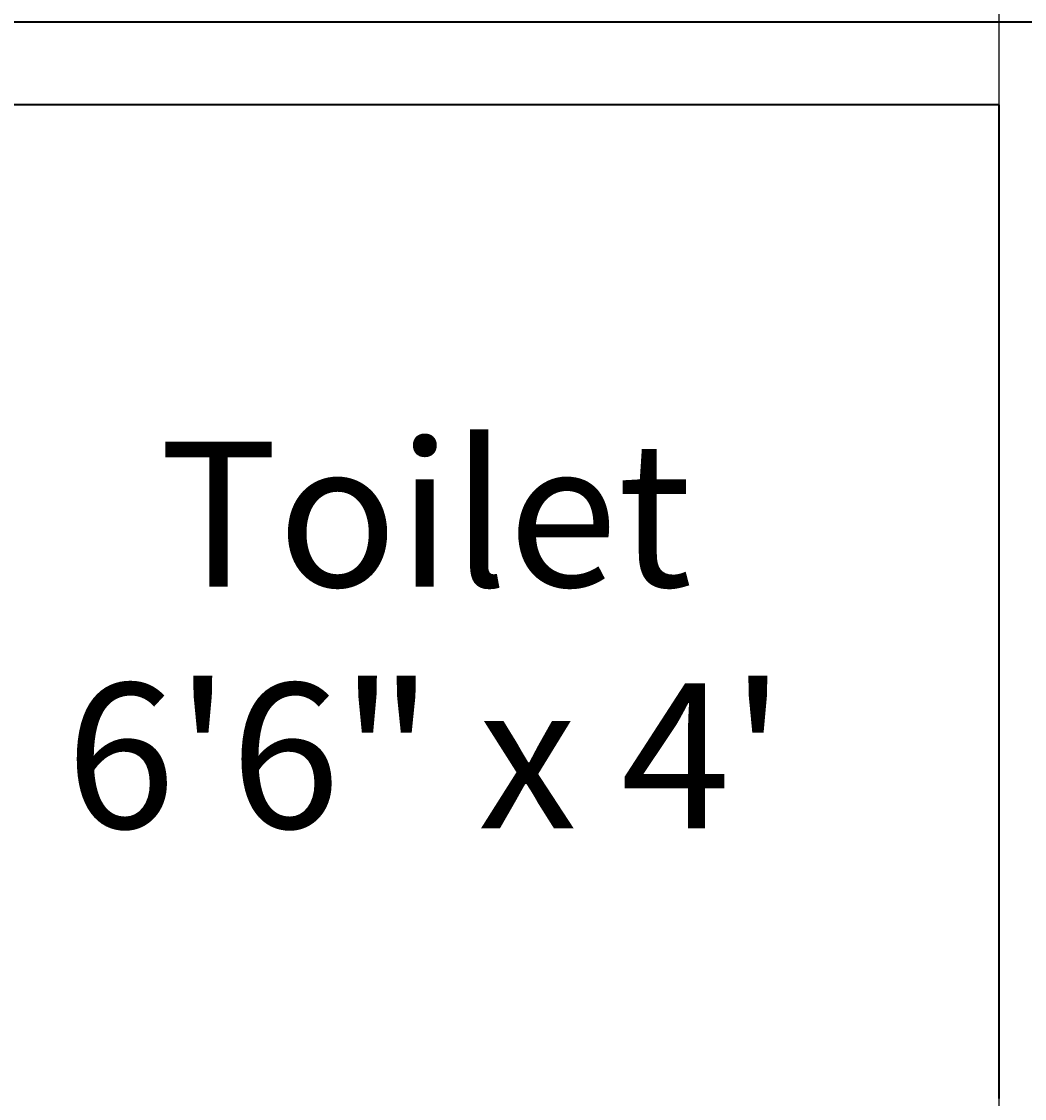
# Model space of a CAD drawing. Units: feet. Extents: x 105 to 1094, y -88 to 588.
# Tile 18 of 59: x 323 to 372, y 302 to 354. Entities that reach past the tile are written whole.
import ezdxf

# ---------------------------------------------------------------- set-up
doc = ezdxf.new("R2010")
doc.units = ezdxf.units.FT
doc.header["$MEASUREMENT"] = 0
for name, color, linetype, lineweight in [('A-ANNO-DIMS', 2, 'Continuous', 18), ('A-AREA-IDEN', 7, 'Continuous', 18), ('A-WALL', 7, 'Continuous', 35)]:
    doc.layers.add(name, color=color, linetype=linetype, lineweight=lineweight)
doc.styles.get("Standard").update_dxf_attribs({"font": 'arial.ttf'})
doc.dimstyles.get("Standard").update_dxf_attribs({"dimtxt": 0.18, "dimasz": 0.18, "dimexe": 0.18, "dimexo": 0.0625, "dimgap": 0.09, "dimtad": 0, "dimtih": 1, "dimtoh": 1, "dimdec": 4, "dimzin": 0, "dimdsep": 46, "dimtxsty": 'Standard', "dimcen": 0.09, "dimadec": 0, "dimazin": 0, "dimtfac": 1, "dimtdec": 4, "dimtofl": 0, "dimtmove": 0, "dimatfit": 3, "dimfxl": 1, "dimtolj": 1, "dimtzin": 0, "dimarcsym": 0})

# ---------------------------------------------------------------- blocks, each defined once
blk = doc.blocks.new('*D21')
at = {"layer": 'A-ANNO-DIMS', "color": 0, "lineweight": -2, "transparency": 16777216}
for p, q in [((849.626, 543.081), (105.458, 543.081)), ((105.638, 542.901), (105.638, 250.263)), ((105.638, -42.739), (105.638, 249.899)), ((849.626, -42.919), (105.458, -42.919))]:
    blk.add_line(p, q, dxfattribs=at)
at = {"layer": 'A-ANNO-DIMS', "color": 0, "transparency": 16777216}
for points in [[(105.608, 542.901), (105.668, 542.901), (105.638, 543.081)], [(105.608, -42.739), (105.668, -42.739), (105.638, -42.919)]]:
    blk.add_solid(points, dxfattribs=at)
at = {"layer": 'Defpoints', "color": 0, "transparency": 16777216}
for p in [(105.638, 543.081), (849.688, 543.081), (849.688, -42.919)]:
    blk.add_point(p, dxfattribs=at)
at = {"layer": 'A-ANNO-DIMS', "color": 0, "transparency": 16777216, "insert": (105.638, 250.081), "char_height": 0.18, "attachment_point": 5}
blk.add_mtext('\\A1;586', dxfattribs=at)
blk = doc.blocks.new('*D33')
at = {"layer": 'A-ANNO-DIMS', "color": 0, "lineweight": -2, "transparency": 16777216}
for p, q in [((646.626, 395.081), (105.458, 395.081)), ((105.638, 394.901), (105.638, 345.263)), ((105.638, 295.261), (105.638, 344.899)), ((646.626, 295.081), (105.458, 295.081))]:
    blk.add_line(p, q, dxfattribs=at)
at = {"layer": 'A-ANNO-DIMS', "color": 0, "transparency": 16777216}
for points in [[(105.608, 394.901), (105.668, 394.901), (105.638, 395.081)], [(105.608, 295.261), (105.668, 295.261), (105.638, 295.081)]]:
    blk.add_solid(points, dxfattribs=at)
at = {"layer": 'Defpoints', "color": 0, "transparency": 16777216}
for p in [(646.688, 395.081), (105.638, 295.081), (646.688, 295.081)]:
    blk.add_point(p, dxfattribs=at)
at = {"layer": 'A-ANNO-DIMS', "color": 0, "transparency": 16777216, "insert": (105.638, 345.081), "char_height": 0.18, "attachment_point": 5}
blk.add_mtext('\\A1;100', dxfattribs=at)
blk = doc.blocks.new('*D39')
at = {"layer": 'A-ANNO-DIMS', "color": 0, "lineweight": -2, "transparency": 16777216}
for p, q in [((294.688, 204.144), (294.688, 588.311)), ((294.868, 588.131), (332.47, 588.131)), ((370.508, 588.131), (332.906, 588.131)), ((370.688, 204.144), (370.688, 588.311))]:
    blk.add_line(p, q, dxfattribs=at)
at = {"layer": 'A-ANNO-DIMS', "color": 0, "transparency": 16777216}
for points in [[(294.868, 588.161), (294.868, 588.101), (294.688, 588.131)], [(370.508, 588.161), (370.508, 588.101), (370.688, 588.131)]]:
    blk.add_solid(points, dxfattribs=at)
at = {"layer": 'Defpoints', "color": 0, "transparency": 16777216}
for p in [(370.688, 588.131), (294.688, 204.081), (370.688, 204.081)]:
    blk.add_point(p, dxfattribs=at)
at = {"layer": 'A-ANNO-DIMS', "color": 0, "transparency": 16777216, "insert": (332.688, 588.131), "char_height": 0.18, "attachment_point": 5}
blk.add_mtext('\\A1;76', dxfattribs=at)
blk = doc.blocks.new('*D51')
at = {"layer": 'A-ANNO-DIMS', "color": 0, "lineweight": -2, "transparency": 16777216}
for p, q in [((432.626, 394.081), (105.458, 394.081)), ((105.638, 393.901), (105.638, 374.263)), ((105.638, 354.261), (105.638, 373.899)), ((426.626, 354.081), (105.458, 354.081))]:
    blk.add_line(p, q, dxfattribs=at)
at = {"layer": 'A-ANNO-DIMS', "color": 0, "transparency": 16777216}
for points in [[(105.608, 393.901), (105.668, 393.901), (105.638, 394.081)], [(105.608, 354.261), (105.668, 354.261), (105.638, 354.081)]]:
    blk.add_solid(points, dxfattribs=at)
at = {"layer": 'Defpoints', "color": 0, "transparency": 16777216}
for p in [(432.688, 394.081), (105.638, 354.081), (426.688, 354.081)]:
    blk.add_point(p, dxfattribs=at)
at = {"layer": 'A-ANNO-DIMS', "color": 0, "transparency": 16777216, "insert": (105.638, 374.081), "char_height": 0.18, "attachment_point": 5}
blk.add_mtext('\\A1;40', dxfattribs=at)

msp = doc.modelspace()

# ---------------------------------------------------------------- linework, layer by layer
at = {"layer": 'A-WALL'}
for p, q in [((374.6883, 354.0812), (288.6883, 354.0812)), ((370.6883, 350.0812), (288.6883, 350.0812)), ((370.6883, 302.0812), (370.6883, 350.0812))]:
    msp.add_line(p, q, dxfattribs=at)

# ---------------------------------------------------------------- texts
at = {"layer": 'A-AREA-IDEN', "insert": (392.1604, 333.8075), "char_height": 7, "attachment_point": 3}
msp.add_mtext_dynamic_manual_height_columns('\\pxqc;Toilet \\P6\'6" x 4\'', width=98.34246, gutter_width=1, heights=[0], dxfattribs=at)

# ---------------------------------------------------------------- dimensions: what is measured, and where the dimension line sits
at = {"layer": 'A-ANNO-DIMS'}
dim = msp.add_linear_dim(base=(370.6883, 588.1312), p1=(294.6883, 204.0812), p2=(370.6883, 204.0812), dimstyle='Standard', override={"dimdec": 0, "dimlfac": 1, "dimrnd": 0, "dimzin": 0, "dimdsep": 46, "dimlunit": 2}, dxfattribs=at)
dim.commit()
dim.dimension.update_dxf_attribs({"geometry": '*D39', "text_midpoint": (332.6883, 588.1312)})
for base, p1, p2, picture, middle in [((105.6383, 543.0812), (849.6883, -42.9188), (849.6883, 543.0812), '*D21', (105.6383, 250.0812)), ((105.6383, 295.0812), (646.6883, 395.0812), (646.6883, 295.0812), '*D33', (105.6383, 345.0812)), ((105.6383, 354.0812), (432.6883, 394.0812), (426.6883, 354.0812), '*D51', (105.6383, 374.0812))]:
    dim = msp.add_linear_dim(base=base, p1=p1, p2=p2, angle=90, dimstyle='Standard', override={"dimdec": 0, "dimlfac": 1, "dimrnd": 0, "dimzin": 0, "dimdsep": 46, "dimlunit": 2}, dxfattribs=at)
    dim.commit()
    dim.dimension.update_dxf_attribs({"geometry": picture, "text_midpoint": middle})

doc.saveas('drawing.dxf')
